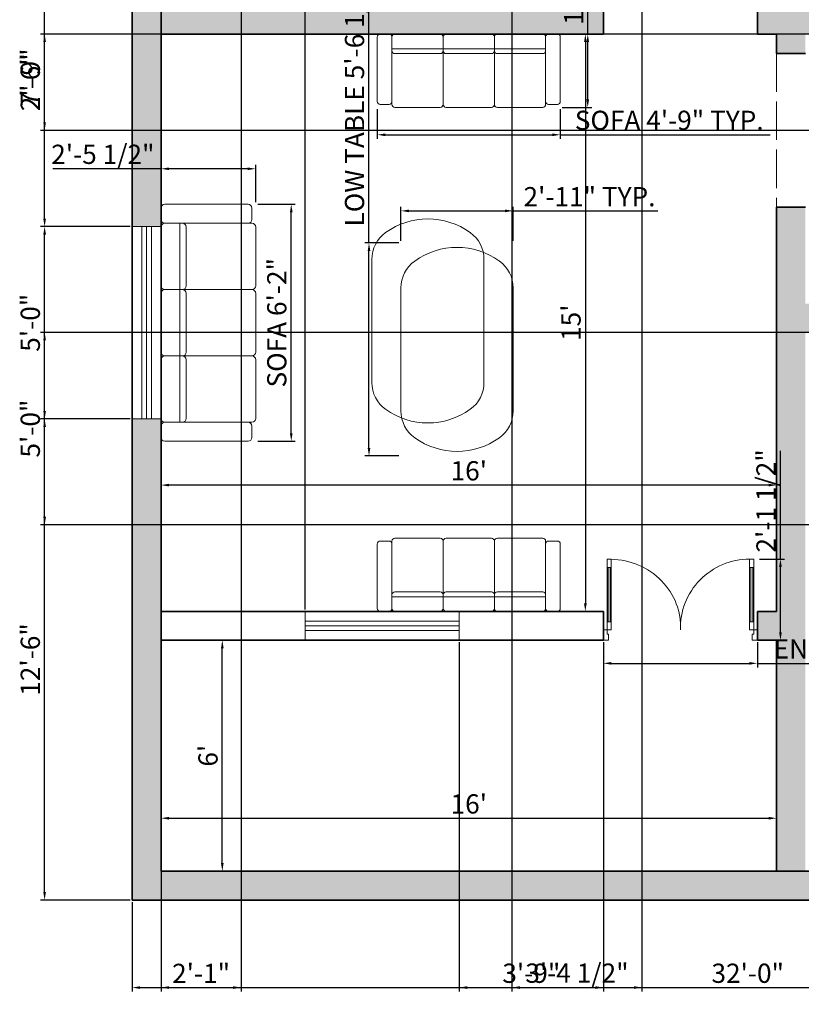
# Model space of a CAD drawing. Units: inches. Extents: x -40 to 424, y -33 to 568.
# Tile 1 of 8: x -35 to 209, y -33 to 275. Entities that reach past the tile are written whole.
import ezdxf

# ---------------------------------------------------------------- set-up
doc = ezdxf.new("R2010")
doc.units = ezdxf.units.IN
doc.linetypes.add('ACAD_ISO02W100', pattern=[15, 12, -3])
for name, color, linetype, lineweight in [('A-ANNO-DIMS', 7, 'Continuous', 18), ('A-DOOR', 7, 'Continuous', 18), ('A-FURN', 7, 'Continuous', 18), ('A-GLAZ', 7, 'Continuous', 18), ('A-WALL-OVHD', 7, 'ACAD_ISO02W100', 18), ('A-WALL-PATT', 30, 'Continuous', 13), ('wall', 7, 'Continuous', 35)]:
    doc.layers.add(name, color=color, linetype=linetype, lineweight=lineweight)
doc.styles.get("Standard").update_dxf_attribs({"font": 'arial.ttf'})
doc.dimstyles.new('ISO-25', dxfattribs={"dimtxt": 6, "dimasz": 2.5, "dimexe": 1.25, "dimexo": 0.625, "dimtad": 1, "dimdec": 1, "dimlunit": 3, "dimtxsty": 'Standard', "dimcen": 2.5, "dimadec": 0, "dimazin": 0, "dimtfac": 1, "dimtdec": 1, "dimtmove": 0, "dimatfit": 3, "dimfxl": 1, "dimarcsym": 0})

# ---------------------------------------------------------------- blocks, each defined once
blk = doc.blocks.new('A$C0A95752C')
for p, q in [((35, 710), (35, 790)), ((35, 790), (75, 790)), ((75, 790), (75, 710)), ((1425, 790), (1425, 710)), ((1465, 790), (1425, 790)), ((1465, 710), (1465, 790)), ((35, 710), (35, 180)), ((75, 710), (35, 710)), ((75, 710), (35, 710)), ((45, 710), (45, 180)), ((65, 710), (45, 710)), ((65, 180), (65, 710)), ((75, 180), (75, 710)), ((1425, 710), (1465, 710)), ((1425, 180), (1425, 710)), ((1425, 710), (1465, 710)), ((1435, 180), (1435, 710)), ((1435, 710), (1455, 710)), ((1455, 710), (1455, 180)), ((1465, 710), (1465, 180)), ((0, 100), (0, 0)), ((35, 100), (0, 100)), ((35, 180), (35, 100)), ((75, 180), (35, 180)), ((35, 180), (75, 180)), ((35, 100), (75, 100)), ((35, 60), (35, 100)), ((45, 180), (65, 180)), ((75, 100), (75, 180)), ((1465, 180), (1425, 180)), ((1425, 100), (1425, 180)), ((1425, 180), (1465, 180)), ((1465, 100), (1425, 100)), ((1455, 180), (1435, 180)), ((1465, 180), (1465, 100)), ((1465, 100), (1500, 100)), ((1465, 60), (1465, 100)), ((1500, 100), (1500, 0)), ((50, 60), (35, 60)), ((50, 50), (50, 60)), ((50, 0), (50, 50)), ((1450, 50), (1450, 60)), ((1450, 60), (1465, 60)), ((1450, 0), (1450, 50)), ((0, 0), (50, 0)), ((1500, 0), (1450, 0))]:
    blk.add_line(p, q)
blk.add_arc((1422.2, 117), 673, 89.76573, 181.44381)
blk.add_ellipse((73.9, 151.1), major_axis=(666.9, -121.7), ratio=0.940794, start_param=0.11153, end_param=1.73917)
blk = doc.blocks.new('A$C0513100E')
for p, q in [((0, 0.768), (0, 0.064)), ((0.032, 0.8), (0.128, 0.8)), ((0.16, 0.768), (0.16, 0.032)), ((0.688, 0.8), (0.192, 0.8)), ((0.72, 0.768), (0.72, 0.032)), ((1.248, 0.8), (0.752, 0.8)), ((1.28, 0.768), (1.28, 0.032)), ((1.808, 0.8), (1.312, 0.8)), ((1.84, 0.032), (1.84, 0.768)), ((1.872, 0.8), (1.968, 0.8)), ((2, 0.064), (2, 0.768)), ((0.72, 0.64), (0.16, 0.64)), ((0.688, 0.5867), (0.192, 0.5867)), ((1.28, 0.64), (0.72, 0.64)), ((1.248, 0.5867), (0.752, 0.5867)), ((1.84, 0.64), (1.28, 0.64)), ((1.808, 0.5867), (1.312, 0.5867)), ((0.72, 0.064), (0.72, 0.4017)), ((1.28, 0.064), (1.28, 0.4017)), ((1.84, 0.064), (1.84, 0.4017)), ((0.032, 0.032), (0.128, 0.032)), ((0.192, 0), (0.688, 0)), ((0.752, 0), (1.248, 0)), ((1.312, 0), (1.808, 0)), ((1.872, 0.032), (1.968, 0.032))]:
    blk.add_line(p, q)
for centre, start, end in [((0.032, 0.768), 90, 180), ((0.128, 0.768), 0, 90), ((0.192, 0.768), 90, 180), ((0.688, 0.768), 0, 90), ((0.752, 0.768), 90, 180), ((1.248, 0.768), 0, 90), ((1.312, 0.768), 90, 180), ((1.808, 0.768), 0, 90), ((1.872, 0.768), 90, 180), ((1.968, 0.768), 0, 90), ((0.192, 0.6187), 180, 270), ((0.688, 0.6187), 270, 0), ((0.752, 0.6187), 180, 270), ((1.248, 0.6187), 270, 0), ((1.312, 0.6187), 180, 270), ((1.808, 0.6187), 270, 0), ((0.032, 0.064), 180, 270), ((0.128, 0.064), 270, 0), ((0.192, 0.032), 180, 270), ((0.688, 0.032), 270, 0), ((0.752, 0.032), 180, 270), ((1.248, 0.032), 270, 0), ((1.312, 0.032), 180, 270), ((1.808, 0.032), 270, 0), ((1.872, 0.064), 180, 270), ((1.968, 0.064), 270, 0)]:
    blk.add_arc(centre, 0.032, start, end)
blk = doc.blocks.new('*D17')
at = {"layer": 'A-ANNO-DIMS', "color": 0, "lineweight": -2, "transparency": 16777216}
for p, q in [((9.63, 81), (29.37, 81)), ((28.12, 11.5), (28.12, 78.5)), ((9.63, 9), (29.37, 9))]:
    blk.add_line(p, q, dxfattribs=at)
at = {"layer": 'A-ANNO-DIMS', "color": 0, "transparency": 16777216}
for points in [[(27.71, 78.5), (28.54, 78.5), (28.12, 81)], [(27.71, 11.5), (28.54, 11.5), (28.12, 9)]]:
    blk.add_solid(points, dxfattribs=at)
at = {"layer": 'Defpoints', "color": 0, "transparency": 16777216}
for p in [(9, 81), (28.12, 81), (9, 9)]:
    blk.add_point(p, dxfattribs=at)
at = {"layer": 'A-ANNO-DIMS', "color": 0, "transparency": 16777216, "insert": (24.43, 45), "char_height": 6, "attachment_point": 5, "rotation": 90}
blk.add_mtext("6'", dxfattribs=at)
blk = doc.blocks.new('*D18')
at = {"layer": 'A-ANNO-DIMS', "color": 0, "lineweight": -2, "transparency": 16777216}
for p, q in [((9, 33.09), (9, 24.25)), ((201, 31.04), (201, 24.25)), ((11.5, 25.5), (198.5, 25.5))]:
    blk.add_line(p, q, dxfattribs=at)
at = {"layer": 'A-ANNO-DIMS', "color": 0, "transparency": 16777216}
for points in [[(11.5, 25.92), (11.5, 25.08), (9, 25.5)], [(198.5, 25.92), (198.5, 25.08), (201, 25.5)]]:
    blk.add_solid(points, dxfattribs=at)
at = {"layer": 'Defpoints', "color": 0, "transparency": 16777216}
for p in [(9, 33.71), (201, 31.66), (201, 25.5)]:
    blk.add_point(p, dxfattribs=at)
at = {"layer": 'A-ANNO-DIMS', "color": 0, "transparency": 16777216, "insert": (105, 29.19), "char_height": 6, "attachment_point": 5}
blk.add_mtext("16'", dxfattribs=at)
blk = doc.blocks.new('*D23')
at = {"layer": 'A-ANNO-DIMS', "color": 0, "lineweight": -2, "transparency": 16777216}
for p, q in [((9, 132.5), (9, 128.12)), ((201, 132.5), (201, 128.12)), ((198.5, 129.37), (11.5, 129.37))]:
    blk.add_line(p, q, dxfattribs=at)
at = {"layer": 'A-ANNO-DIMS', "color": 0, "transparency": 16777216}
for points in [[(11.5, 129.79), (11.5, 128.96), (9, 129.37)], [(198.5, 129.79), (198.5, 128.96), (201, 129.37)]]:
    blk.add_solid(points, dxfattribs=at)
at = {"layer": 'Defpoints', "color": 0, "transparency": 16777216}
for p in [(9, 133.12), (201, 133.12), (9, 129.37)]:
    blk.add_point(p, dxfattribs=at)
at = {"layer": 'A-ANNO-DIMS', "color": 0, "transparency": 16777216, "insert": (105, 133.06), "char_height": 6, "attachment_point": 5}
blk.add_mtext("16'", dxfattribs=at)
blk = doc.blocks.new('*D24')
at = {"layer": 'A-ANNO-DIMS', "color": 0, "lineweight": -2, "transparency": 16777216}
for p, q in [((146.38, 270), (140.1, 270)), ((141.35, 267.5), (141.35, 92.5)), ((142.23, 90), (140.1, 90))]:
    blk.add_line(p, q, dxfattribs=at)
at = {"layer": 'A-ANNO-DIMS', "color": 0, "transparency": 16777216}
for points in [[(140.94, 267.5), (141.77, 267.5), (141.35, 270)], [(140.94, 92.5), (141.77, 92.5), (141.35, 90)]]:
    blk.add_solid(points, dxfattribs=at)
at = {"layer": 'Defpoints', "color": 0, "transparency": 16777216}
for p in [(147, 270), (141.35, 90), (142.85, 90)]:
    blk.add_point(p, dxfattribs=at)
at = {"layer": 'A-ANNO-DIMS', "color": 0, "transparency": 16777216, "insert": (137.67, 180), "char_height": 6, "attachment_point": 5, "rotation": 90}
blk.add_mtext("15'", dxfattribs=at)
blk = doc.blocks.new('WIN-48IN')
for p, q in [((0, 0), (0, 9)), ((48, 0), (48, 9)), ((0, 6), (48, 6)), ((0, 4.5), (48, 4.5)), ((0, 3), (48, 3))]:
    blk.add_line(p, q)
blk = doc.blocks.new('TABLE-LOW-OBLONG')
for points in [[(35, 20.37), (35, 50.99, 0.241531), (30.71, 59.36, 0.321887), (4.29, 59.36, 0.241531), (0, 50.99), (0, 20.37)], [(35, 43.24), (35, 12.61, -0.241531), (30.71, 4.25, -0.321887), (4.29, 4.25, -0.241531), (0, 12.61), (0, 43.24)]]:
    blk.add_lwpolyline(points, format="xyb")
blk = doc.blocks.new('*D51')
at = {"layer": 'A-ANNO-DIMS', "color": 0, "lineweight": -2, "transparency": 16777216}
for p, q in [((147, 80.37), (147, 72.55)), ((195, 80.37), (195, 72.55)), ((149.5, 73.8), (192.5, 73.8)), ((195, 73.8), (272.6, 73.8))]:
    blk.add_line(p, q, dxfattribs=at)
at = {"layer": 'A-ANNO-DIMS', "color": 0, "transparency": 16777216}
for points in [[(149.5, 74.22), (149.5, 73.38), (147, 73.8)], [(192.5, 74.22), (192.5, 73.38), (195, 73.8)]]:
    blk.add_solid(points, dxfattribs=at)
at = {"layer": 'Defpoints', "color": 0, "transparency": 16777216}
for p in [(147, 81), (195, 81), (195, 73.8)]:
    blk.add_point(p, dxfattribs=at)
at = {"layer": 'A-ANNO-DIMS', "color": 0, "transparency": 16777216, "insert": (235.05, 77.53), "char_height": 6, "attachment_point": 5}
blk.add_mtext('ENTRY DOOR 4\'-0"', dxfattribs=at)
blk = doc.blocks.new('*D52')
at = {"layer": 'A-ANNO-DIMS', "color": 0, "lineweight": -2, "transparency": 16777216}
for p, q in [((202.2, 106.3), (202.2, 140.09)), ((195.63, 106.3), (203.45, 106.3)), ((202.2, 83.5), (202.2, 103.8)), ((195.63, 81), (203.45, 81))]:
    blk.add_line(p, q, dxfattribs=at)
at = {"layer": 'A-ANNO-DIMS', "color": 0, "transparency": 16777216}
for points in [[(201.78, 103.8), (202.62, 103.8), (202.2, 106.3)], [(201.78, 83.5), (202.62, 83.5), (202.2, 81)]]:
    blk.add_solid(points, dxfattribs=at)
at = {"layer": 'Defpoints', "color": 0, "transparency": 16777216}
for p in [(195, 106.3), (202.2, 106.3), (195, 81)]:
    blk.add_point(p, dxfattribs=at)
at = {"layer": 'A-ANNO-DIMS', "color": 0, "transparency": 16777216, "insert": (198.47, 124.45), "char_height": 6, "attachment_point": 5, "rotation": 90}
blk.add_mtext('2\'-1 1/2"', dxfattribs=at)
blk = doc.blocks.new('*D53')
at = {"layer": 'A-ANNO-DIMS', "color": 0, "lineweight": -2, "transparency": 16777216}
for p, q in [((39.17, 216.93), (50.87, 216.93)), ((49.62, 145.57), (49.62, 214.43)), ((39.17, 143.07), (50.87, 143.07))]:
    blk.add_line(p, q, dxfattribs=at)
at = {"layer": 'A-ANNO-DIMS', "color": 0, "transparency": 16777216}
for points in [[(49.21, 214.43), (50.04, 214.43), (49.62, 216.93)], [(49.21, 145.57), (50.04, 145.57), (49.62, 143.07)]]:
    blk.add_solid(points, dxfattribs=at)
at = {"layer": 'Defpoints', "color": 0, "transparency": 16777216}
for p in [(38.54, 216.93), (49.62, 216.93), (38.54, 143.07)]:
    blk.add_point(p, dxfattribs=at)
at = {"layer": 'A-ANNO-DIMS', "color": 0, "transparency": 16777216, "insert": (45.89, 180), "char_height": 6, "attachment_point": 5, "rotation": 90}
blk.add_mtext('SOFA 6\'-2"', dxfattribs=at)
blk = doc.blocks.new('*D54')
at = {"layer": 'A-ANNO-DIMS', "color": 0, "lineweight": -2, "transparency": 16777216}
for p, q in [((9, 228.01), (-24.78, 228.01)), ((9, 217.55), (9, 229.26)), ((36.04, 228.01), (11.5, 228.01)), ((38.54, 217.55), (38.54, 229.26))]:
    blk.add_line(p, q, dxfattribs=at)
at = {"layer": 'A-ANNO-DIMS', "color": 0, "transparency": 16777216}
for points in [[(11.5, 228.42), (11.5, 227.59), (9, 228.01)], [(36.04, 228.42), (36.04, 227.59), (38.54, 228.01)]]:
    blk.add_solid(points, dxfattribs=at)
at = {"layer": 'Defpoints', "color": 0, "transparency": 16777216}
for p in [(9, 228.01), (9, 216.93), (38.54, 216.93)]:
    blk.add_point(p, dxfattribs=at)
at = {"layer": 'A-ANNO-DIMS', "color": 0, "transparency": 16777216, "insert": (-9.14, 231.74), "char_height": 6, "attachment_point": 5}
blk.add_mtext('2\'-5 1/2"', dxfattribs=at)
blk = doc.blocks.new('*D55')
at = {"layer": 'A-ANNO-DIMS', "color": 0, "lineweight": -2, "transparency": 16777216}
for p, q in [((76.46, 246.55), (76.46, 237.36)), ((133.54, 246.55), (133.54, 237.36)), ((78.96, 238.61), (131.04, 238.61)), ((133.54, 238.61), (198.98, 238.61))]:
    blk.add_line(p, q, dxfattribs=at)
at = {"layer": 'A-ANNO-DIMS', "color": 0, "transparency": 16777216}
for points in [[(78.96, 239.03), (78.96, 238.19), (76.46, 238.61)], [(131.04, 239.03), (131.04, 238.19), (133.54, 238.61)]]:
    blk.add_solid(points, dxfattribs=at)
at = {"layer": 'Defpoints', "color": 0, "transparency": 16777216}
for p in [(76.46, 247.17), (133.54, 247.17), (133.54, 238.61)]:
    blk.add_point(p, dxfattribs=at)
at = {"layer": 'A-ANNO-DIMS', "color": 0, "transparency": 16777216, "insert": (167.51, 242.34), "char_height": 6, "attachment_point": 5}
blk.add_mtext('SOFA 4\'-9" TYP.', dxfattribs=at)
blk = doc.blocks.new('*D56')
at = {"layer": 'A-ANNO-DIMS', "color": 0, "lineweight": -2, "transparency": 16777216}
for p, q in [((142.1, 270), (142.1, 314.42)), ((134.16, 270), (143.35, 270)), ((142.1, 249.67), (142.1, 267.5)), ((134.16, 247.17), (143.35, 247.17))]:
    blk.add_line(p, q, dxfattribs=at)
at = {"layer": 'A-ANNO-DIMS', "color": 0, "transparency": 16777216}
for points in [[(141.68, 267.5), (142.51, 267.5), (142.1, 270)], [(141.68, 249.67), (142.51, 249.67), (142.1, 247.17)]]:
    blk.add_solid(points, dxfattribs=at)
at = {"layer": 'Defpoints', "color": 0, "transparency": 16777216}
for p in [(133.54, 270), (142.1, 270), (133.54, 247.17)]:
    blk.add_point(p, dxfattribs=at)
at = {"layer": 'A-ANNO-DIMS', "color": 0, "transparency": 16777216, "insert": (138.46, 293.46), "char_height": 6, "attachment_point": 5, "rotation": 90}
blk.add_mtext('1\'-11" TYP.', dxfattribs=at)
blk = doc.blocks.new('*D59')
at = {"layer": 'A-ANNO-DIMS', "color": 0, "lineweight": -2, "transparency": 16777216}
for p, q in [((73.87, 204.92), (73.87, 309.26)), ((83.22, 204.92), (72.62, 204.92)), ((73.87, 140.98), (73.87, 202.42)), ((83.22, 138.48), (72.62, 138.48))]:
    blk.add_line(p, q, dxfattribs=at)
at = {"layer": 'A-ANNO-DIMS', "color": 0, "transparency": 16777216}
for points in [[(73.46, 202.42), (74.29, 202.42), (73.87, 204.92)], [(73.46, 140.98), (74.29, 140.98), (73.87, 138.48)]]:
    blk.add_solid(points, dxfattribs=at)
at = {"layer": 'Defpoints', "color": 0, "transparency": 16777216}
for p in [(73.87, 204.92), (83.84, 204.92), (83.84, 138.48)]:
    blk.add_point(p, dxfattribs=at)
at = {"layer": 'A-ANNO-DIMS', "color": 0, "transparency": 16777216, "insert": (70.14, 258.34), "char_height": 6, "attachment_point": 5, "rotation": 90}
blk.add_mtext('LOW TABLE 5\'-6 1/2" TYP.', dxfattribs=at)
blk = doc.blocks.new('*D60')
at = {"layer": 'A-ANNO-DIMS', "color": 0, "lineweight": -2, "transparency": 16777216}
for p, q in [((83.84, 205.55), (83.84, 216.14)), ((118.84, 205.55), (118.84, 216.14)), ((86.34, 214.89), (116.34, 214.89)), ((118.84, 214.89), (163.93, 214.89))]:
    blk.add_line(p, q, dxfattribs=at)
at = {"layer": 'A-ANNO-DIMS', "color": 0, "transparency": 16777216}
for points in [[(86.34, 215.3), (86.34, 214.47), (83.84, 214.89)], [(116.34, 215.3), (116.34, 214.47), (118.84, 214.89)]]:
    blk.add_solid(points, dxfattribs=at)
at = {"layer": 'Defpoints', "color": 0, "transparency": 16777216}
for p in [(118.84, 214.89), (83.84, 204.92), (118.84, 204.92)]:
    blk.add_point(p, dxfattribs=at)
at = {"layer": 'A-ANNO-DIMS', "color": 0, "transparency": 16777216, "insert": (142.64, 218.53), "char_height": 6, "attachment_point": 5}
blk.add_mtext('2\'-11" TYP.', dxfattribs=at)
blk = doc.blocks.new('*D79')
at = {"layer": 'A-ANNO-DIMS', "color": 0, "lineweight": -2, "transparency": 16777216}
for p, q in [((0, -0.62), (0, -28.55)), ((384, -0.62), (384, -28.55)), ((2.5, -27.3), (381.5, -27.3))]:
    blk.add_line(p, q, dxfattribs=at)
at = {"layer": 'A-ANNO-DIMS', "color": 0, "transparency": 16777216}
for points in [[(2.5, -26.88), (2.5, -27.72), (0, -27.3)], [(381.5, -26.88), (381.5, -27.72), (384, -27.3)]]:
    blk.add_solid(points, dxfattribs=at)
at = {"layer": 'Defpoints', "color": 0, "transparency": 16777216}
for p in [(0, 0), (384, 0), (384, -27.3)]:
    blk.add_point(p, dxfattribs=at)
at = {"layer": 'A-ANNO-DIMS', "color": 0, "transparency": 16777216, "insert": (192, -23.61), "char_height": 6, "attachment_point": 5}
blk.add_mtext('32\'-0"', dxfattribs=at)
blk = doc.blocks.new('*D81')
at = {"layer": 'A-ANNO-DIMS', "color": 0, "lineweight": -2, "transparency": 16777216}
for p, q in [((-0.63, 210), (-28.55, 210)), ((-27.3, 152.5), (-27.3, 207.5)), ((-0.63, 150), (-28.55, 150))]:
    blk.add_line(p, q, dxfattribs=at)
at = {"layer": 'A-ANNO-DIMS', "color": 0, "transparency": 16777216}
for points in [[(-27.72, 207.5), (-26.88, 207.5), (-27.3, 210)], [(-27.72, 152.5), (-26.88, 152.5), (-27.3, 150)]]:
    blk.add_solid(points, dxfattribs=at)
at = {"layer": 'Defpoints', "color": 0, "transparency": 16777216}
for p in [(-27.3, 210), (0, 210), (0, 150)]:
    blk.add_point(p, dxfattribs=at)
at = {"layer": 'A-ANNO-DIMS', "color": 0, "transparency": 16777216, "insert": (-30.99, 180), "char_height": 6, "attachment_point": 5, "rotation": 90}
blk.add_mtext('5\'-0"', dxfattribs=at)
blk = doc.blocks.new('*D82')
at = {"layer": 'A-ANNO-DIMS', "color": 0, "lineweight": -2, "transparency": 16777216}
for p, q in [((-0.63, 150), (-28.55, 150)), ((-27.3, 2.5), (-27.3, 147.5)), ((-0.63, 0), (-28.55, 0))]:
    blk.add_line(p, q, dxfattribs=at)
at = {"layer": 'A-ANNO-DIMS', "color": 0, "transparency": 16777216}
for points in [[(-27.72, 147.5), (-26.88, 147.5), (-27.3, 150)], [(-27.72, 2.5), (-26.88, 2.5), (-27.3, 0)]]:
    blk.add_solid(points, dxfattribs=at)
at = {"layer": 'Defpoints', "color": 0, "transparency": 16777216}
for p in [(-27.3, 150), (0, 150), (0, 0)]:
    blk.add_point(p, dxfattribs=at)
at = {"layer": 'A-ANNO-DIMS', "color": 0, "transparency": 16777216, "insert": (-30.99, 75), "char_height": 6, "attachment_point": 5, "rotation": 90}
blk.add_mtext('12\'-6"', dxfattribs=at)
blk = doc.blocks.new('*D83')
at = {"layer": 'A-ANNO-DIMS', "color": 0, "lineweight": -2, "transparency": 16777216}
for p, q in [((-0.63, 303), (-28.55, 303)), ((-27.3, 212.5), (-27.3, 300.5)), ((-0.63, 210), (-28.55, 210))]:
    blk.add_line(p, q, dxfattribs=at)
at = {"layer": 'A-ANNO-DIMS', "color": 0, "transparency": 16777216}
for points in [[(-27.72, 300.5), (-26.88, 300.5), (-27.3, 303)], [(-27.72, 212.5), (-26.88, 212.5), (-27.3, 210)]]:
    blk.add_solid(points, dxfattribs=at)
at = {"layer": 'Defpoints', "color": 0, "transparency": 16777216}
for p in [(-27.3, 303), (0, 303), (0, 210)]:
    blk.add_point(p, dxfattribs=at)
at = {"layer": 'A-ANNO-DIMS', "color": 0, "transparency": 16777216, "insert": (-30.99, 256.5), "char_height": 6, "attachment_point": 5, "rotation": 90}
blk.add_mtext('7\'-9"', dxfattribs=at)
blk = doc.blocks.new('*D87')
at = {"layer": 'A-ANNO-DIMS', "color": 0, "lineweight": -2, "transparency": 16777216}
for p, q in [((374.38, 177), (-28.55, 177)), ((-27.3, 119.5), (-27.3, 174.5)), ((374.38, 117), (-28.55, 117))]:
    blk.add_line(p, q, dxfattribs=at)
at = {"layer": 'A-ANNO-DIMS', "color": 0, "transparency": 16777216}
for points in [[(-27.72, 174.5), (-26.88, 174.5), (-27.3, 177)], [(-27.72, 119.5), (-26.88, 119.5), (-27.3, 117)]]:
    blk.add_solid(points, dxfattribs=at)
at = {"layer": 'Defpoints', "color": 0, "transparency": 16777216}
for p in [(-27.3, 177), (375, 177), (375, 117)]:
    blk.add_point(p, dxfattribs=at)
at = {"layer": 'A-ANNO-DIMS', "color": 0, "transparency": 16777216, "insert": (-30.99, 147), "char_height": 6, "attachment_point": 5, "rotation": 90}
blk.add_mtext('5\'-0"', dxfattribs=at)
blk = doc.blocks.new('*D88')
at = {"layer": 'A-ANNO-DIMS', "color": 0, "lineweight": -2, "transparency": 16777216}
for p, q in [((374.38, 270), (-28.55, 270)), ((-27.3, 242.5), (-27.3, 267.5)), ((374.38, 240), (-28.55, 240))]:
    blk.add_line(p, q, dxfattribs=at)
at = {"layer": 'A-ANNO-DIMS', "color": 0, "transparency": 16777216}
for points in [[(-27.72, 267.5), (-26.88, 267.5), (-27.3, 270)], [(-27.72, 242.5), (-26.88, 242.5), (-27.3, 240)]]:
    blk.add_solid(points, dxfattribs=at)
at = {"layer": 'Defpoints', "color": 0, "transparency": 16777216}
for p in [(-27.3, 270), (375, 270), (375, 240)]:
    blk.add_point(p, dxfattribs=at)
at = {"layer": 'A-ANNO-DIMS', "color": 0, "transparency": 16777216, "insert": (-30.99, 255), "char_height": 6, "attachment_point": 5, "rotation": 90}
blk.add_mtext('2\'-6"', dxfattribs=at)
blk = doc.blocks.new('*D90')
at = {"layer": 'A-ANNO-DIMS', "color": 0, "lineweight": -2, "transparency": 16777216}
for p, q in [((102, 80.37), (102, -28.55)), ((147, 80.37), (147, -28.55)), ((104.5, -27.3), (144.5, -27.3))]:
    blk.add_line(p, q, dxfattribs=at)
at = {"layer": 'A-ANNO-DIMS', "color": 0, "transparency": 16777216}
for points in [[(104.5, -26.88), (104.5, -27.72), (102, -27.3)], [(144.5, -26.88), (144.5, -27.72), (147, -27.3)]]:
    blk.add_solid(points, dxfattribs=at)
at = {"layer": 'Defpoints', "color": 0, "transparency": 16777216}
for p in [(102, 81), (147, 81), (147, -27.3)]:
    blk.add_point(p, dxfattribs=at)
at = {"layer": 'A-ANNO-DIMS', "color": 0, "transparency": 16777216, "insert": (124.5, -23.61), "char_height": 6, "attachment_point": 5}
blk.add_mtext('3\'-9"', dxfattribs=at)
blk = doc.blocks.new('*D91')
at = {"layer": 'A-ANNO-DIMS', "color": 0, "lineweight": -2, "transparency": 16777216}
for p, q in [((9, 90.62), (9, 556.55)), ((54, 90.62), (54, 556.55)), ((11.5, 555.3), (51.5, 555.3))]:
    blk.add_line(p, q, dxfattribs=at)
at = {"layer": 'A-ANNO-DIMS', "color": 0, "transparency": 16777216}
for points in [[(11.5, 555.72), (11.5, 554.88), (9, 555.3)], [(51.5, 555.72), (51.5, 554.88), (54, 555.3)]]:
    blk.add_solid(points, dxfattribs=at)
at = {"layer": 'Defpoints', "color": 0, "transparency": 16777216}
for p in [(54, 555.3), (9, 90), (54, 90)]:
    blk.add_point(p, dxfattribs=at)
at = {"layer": 'A-ANNO-DIMS', "color": 0, "transparency": 16777216, "insert": (31.5, 558.99), "char_height": 6, "attachment_point": 5}
blk.add_mtext('3\'-9"', dxfattribs=at)
blk = doc.blocks.new('*D92')
at = {"layer": 'A-ANNO-DIMS', "color": 0, "lineweight": -2, "transparency": 16777216}
for p, q in [((118.47, 470.38), (118.47, -28.55)), ((159, 470.38), (159, -28.55)), ((120.97, -27.3), (156.5, -27.3))]:
    blk.add_line(p, q, dxfattribs=at)
at = {"layer": 'A-ANNO-DIMS', "color": 0, "transparency": 16777216}
for points in [[(120.97, -26.88), (120.97, -27.72), (118.47, -27.3)], [(156.5, -26.88), (156.5, -27.72), (159, -27.3)]]:
    blk.add_solid(points, dxfattribs=at)
at = {"layer": 'Defpoints', "color": 0, "transparency": 16777216}
for p in [(118.47, 471), (159, 471), (159, -27.3)]:
    blk.add_point(p, dxfattribs=at)
at = {"layer": 'A-ANNO-DIMS', "color": 0, "transparency": 16777216, "insert": (138.73, -23.57), "char_height": 6, "attachment_point": 5}
blk.add_mtext('3\'-4 1/2"', dxfattribs=at)
blk = doc.blocks.new('*D101')
at = {"layer": 'A-ANNO-DIMS', "color": 0, "lineweight": -2, "transparency": 16777216}
for p, q in [((9, 357.82), (9, -28.55)), ((34, 357.82), (34, -28.55)), ((11.5, -27.3), (31.5, -27.3))]:
    blk.add_line(p, q, dxfattribs=at)
at = {"layer": 'A-ANNO-DIMS', "color": 0, "transparency": 16777216}
for points in [[(11.5, -26.88), (11.5, -27.72), (9, -27.3)], [(31.5, -26.88), (31.5, -27.72), (34, -27.3)]]:
    blk.add_solid(points, dxfattribs=at)
at = {"layer": 'Defpoints', "color": 0, "transparency": 16777216}
for p in [(9, 358.44), (34, 358.44), (34, -27.3)]:
    blk.add_point(p, dxfattribs=at)
at = {"layer": 'A-ANNO-DIMS', "color": 0, "transparency": 16777216, "insert": (21.5, -23.66), "char_height": 6, "attachment_point": 5}
blk.add_mtext('2\'-1"', dxfattribs=at)

msp = doc.modelspace()

# ---------------------------------------------------------------- hatches: boundary and pattern name
at = {"layer": 'A-WALL-PATT'}
h = msp.add_hatch(color=256, dxfattribs=at)
h.dxf.hatch_style = 1
h.paths.add_polyline_path([(9, 399), (0, 399), (0, 351), (9, 351)])
h.paths.add_polyline_path([(9, 303), (0, 303), (0, 210), (9, 210)])
h.paths.add_polyline_path([(9, 150), (0, 150), (0, 0), (384, 0), (384, 69), (375, 69), (375, 62.24), (375, 9), (9, 9)])
h.paths.add_polyline_path([(210, 177), (216, 177), (216, 186), (210, 186), (210, 216), (201, 216), (201, 90), (195, 90), (195, 81), (201, 81), (201, 9), (210, 9)])
h.paths.add_polyline_path([(384, 216), (375, 216), (375, 117), (384, 117)])
h.paths.add_polyline_path([(384, 298.5), (375, 298.5), (375, 279), (375, 240), (384, 240)])
h.paths.add_polyline_path([(384, 417), (375, 417), (375, 334.5), (384, 334.5)])
h.paths.add_polyline_path([(384, 528), (216, 528), (216, 519), (375, 519), (375, 465), (384, 465)])
h.paths.add_polyline_path([(192, 528), (0, 528), (0, 511.5), (9, 511.5), (9, 519), (192, 519)])
h.paths.add_polyline_path([(9, 487.5), (0, 487.5), (0, 447), (9, 447)])
h.paths.add_polyline_path([(111, 480), (9, 480), (9, 471), (111, 471)])
h.paths.add_polyline_path([(174, 519), (165, 519), (165, 354), (174, 354)])
h.paths.add_polyline_path([(243, 426), (237.86, 426), (234, 426), (234, 420), (174, 420), (174, 411), (234, 411), (234, 405), (239.14, 405), (243, 405)])
h.paths.add_polyline_path([(243, 519), (234, 519), (234, 460.14, -0.031638), (237.86, 460.2), (237.86, 462), (243, 462)])
h.paths.add_polyline_path([(243, 369), (234, 369), (234, 354), (375, 354), (375, 363), (243, 363)])
h.paths.add_polyline_path([(375, 279), (195, 279), (195, 270), (201, 270), (201, 264), (210, 264), (210, 270), (375, 270)])
h.paths.add_polyline_path([(291, 270), (282, 270), (282, 222), (286.29, 222), (291, 222)])
h.paths.add_polyline_path([(375, 186), (291, 186), (291, 192), (282, 192), (282, 186), (252, 186), (252, 180.86), (252, 177), (375, 177)])
h.paths.add_polyline_path([(147, 279), (9, 279), (9, 270), (147, 270)])

# ---------------------------------------------------------------- linework, layer by layer
at = {"layer": 'A-GLAZ'}
for p, q in [((0, 210), (9, 210)), ((3, 210), (3, 150)), ((4.5, 210), (4.5, 150)), ((6, 210), (6, 150)), ((0, 150), (9, 150))]:
    msp.add_line(p, q, dxfattribs=at)
at = {"layer": 'A-WALL-OVHD'}
for p, q in [((195, 270), (147, 270)), ((201, 264), (201, 216))]:
    msp.add_line(p, q, dxfattribs=at)
at = {"layer": 'wall'}
for p, q in [((9, 519), (9, 9)), ((147, 279), (147, 270)), ((195, 279), (195, 270)), ((9, 270), (147, 270)), ((195, 270), (201, 270)), ((201, 270), (201, 264)), ((201, 264), (210, 264)), ((201, 216), (210, 216)), ((201, 216), (201, 90)), ((9, 90), (147, 90)), ((147, 90), (147, 81)), ((195, 90), (195, 81)), ((195, 90), (201, 90)), ((9, 81), (147, 81)), ((195, 81), (201, 81)), ((201, 81), (201, 9)), ((9, 9), (375, 9))]:
    msp.add_line(p, q, dxfattribs=at)
msp.add_lwpolyline([(0, 0), (384, 0), (384, 528), (0, 528)], close=True, dxfattribs=at)

# ---------------------------------------------------------------- block references
at = {"layer": 'A-DOOR', "xscale": 0.032, "yscale": 0.032, "zscale": 0.032}
msp.add_blockref('A$C0A95752C', (147, 81), dxfattribs=at)
at = {"layer": 'A-FURN', "xscale": 28.53662023476671, "yscale": 28.53662023476671, "zscale": 28.53662023476671}
msp.add_blockref('A$C0513100E', (76.46, 247.17), dxfattribs=at)
at = {"layer": 'A-FURN'}
for p, xscale, yscale, zscale, rotation in [((38.54, 143.07), 36.9291377736036, 36.9291377736036, 36.9291377736036, 90), ((76.46, 112.83), -28.53662023476671, 28.53662023476671, 28.53662023476671, 180)]:
    msp.add_blockref('A$C0513100E', p, dxfattribs=dict(at, xscale=xscale, yscale=yscale, zscale=zscale, rotation=rotation))
for p in [(74.74, 148.76), (83.84, 139.89)]:
    msp.add_blockref('TABLE-LOW-OBLONG', p, dxfattribs=at)
at = {"layer": 'A-GLAZ'}
msp.add_blockref('WIN-48IN', (54, 81), dxfattribs=at)

# ---------------------------------------------------------------- dimensions: what is measured, and where the dimension line sits
at = {"layer": 'A-ANNO-DIMS'}
for base, p1, p2, override, picture, middle in [((54, 555.3), (9, 90), (54, 90), {"dimdec": 1, "dimlfac": 1, "dimrnd": 0, "dimzin": 1, "dimdsep": 46, "dimlunit": 4, "dimfrac": 2}, '*D91', (31.5, 558.99)), ((159, -27.3), (118.47, 471), (159, 471), {"dimdec": 1, "dimlfac": 1, "dimrnd": 0, "dimzin": 1, "dimdsep": 46, "dimlunit": 4, "dimfrac": 2}, '*D92', (138.73, -23.57)), ((34, -27.3), (9, 358.44), (34, 358.44), {"dimdec": 1, "dimlfac": 1, "dimrnd": 0, "dimzin": 1, "dimdsep": 46, "dimlunit": 4, "dimfrac": 2}, '*D101', (21.5, -23.66)), ((147, -27.3), (102, 81), (147, 81), {"dimdec": 1, "dimlfac": 1, "dimrnd": 0, "dimzin": 1, "dimdsep": 46, "dimlunit": 4, "dimfrac": 2}, '*D90', (124.5, -23.61)), ((201, 25.5), (9, 33.71), (201, 31.66), {"dimclrd": 0, "dimclre": 0, "dimclrt": 0}, '*D18', (105, 29.19)), ((384, -27.3), (0, 0), (384, 0), {"dimdec": 1, "dimlfac": 1, "dimrnd": 0, "dimzin": 1, "dimdsep": 46, "dimlunit": 4, "dimfrac": 2}, '*D79', (192, -23.61))]:
    dim = msp.add_linear_dim(base=base, p1=p1, p2=p2, dimstyle='ISO-25', override=override, dxfattribs=at)
    dim.commit()
    dim.dimension.update_dxf_attribs({"geometry": picture, "text_midpoint": middle})
for base, p1, p2, text, picture, middle in [((142.1, 270), (133.54, 247.17), (133.54, 270), '<> TYP.', '*D56', (138.46, 293.46)), ((73.87, 204.92), (83.84, 138.48), (83.84, 204.92), 'LOW TABLE <> TYP.', '*D59', (70.14, 258.34)), ((49.62, 216.93), (38.54, 143.07), (38.54, 216.93), 'SOFA <>', '*D53', (45.89, 180))]:
    dim = msp.add_linear_dim(base=base, p1=p1, p2=p2, angle=90, text=text, dimstyle='ISO-25', override={"dimdec": 1, "dimlfac": 1, "dimrnd": 0, "dimzin": 1, "dimdsep": 46, "dimlunit": 4, "dimfrac": 2}, dxfattribs=at)
    dim.commit()
    dim.dimension.update_dxf_attribs({"geometry": picture, "text_midpoint": middle})
for base, p1, p2, angle, override, picture, middle in [((-27.3, 303), (0, 210), (0, 303), 90, {"dimdec": 1, "dimlfac": 1, "dimrnd": 0, "dimzin": 1, "dimdsep": 46, "dimlunit": 4, "dimfrac": 2}, '*D83', (-30.99, 256.5)), ((-27.3, 270), (375, 240), (375, 270), 90, {"dimdec": 1, "dimlfac": 1, "dimrnd": 0, "dimzin": 1, "dimdsep": 46, "dimlunit": 4, "dimfrac": 2}, '*D88', (-30.99, 255)), ((141.35, 90), (147, 270), (142.85, 90), 90, {"dimclrd": 0, "dimclre": 0, "dimclrt": 0}, '*D24', (137.67, 180)), ((9, 228.01), (38.54, 216.93), (9, 216.93), 180, {"dimdec": 1, "dimlfac": 1, "dimrnd": 0, "dimzin": 1, "dimdsep": 46, "dimlunit": 4, "dimfrac": 2}, '*D54', (-9.14, 231.74)), ((-27.3, 210), (0, 150), (0, 210), 90, {"dimdec": 1, "dimlfac": 1, "dimrnd": 0, "dimzin": 1, "dimdsep": 46, "dimlunit": 4, "dimfrac": 2}, '*D81', (-30.99, 180)), ((-27.3, 177), (375, 117), (375, 177), 90, {"dimdec": 1, "dimlfac": 1, "dimrnd": 0, "dimzin": 1, "dimdsep": 46, "dimlunit": 4, "dimfrac": 2}, '*D87', (-30.99, 147)), ((-27.3, 150), (0, 0), (0, 150), 90, {"dimdec": 1, "dimlfac": 1, "dimrnd": 0, "dimzin": 1, "dimdsep": 46, "dimlunit": 4, "dimfrac": 2}, '*D82', (-30.99, 75)), ((202.2, 106.3), (195, 81), (195, 106.3), 90, {"dimdec": 1, "dimlfac": 1, "dimrnd": 0, "dimzin": 1, "dimdsep": 46, "dimlunit": 4, "dimfrac": 2}, '*D52', (198.47, 124.45)), ((28.12, 81), (9, 9), (9, 81), 90, {"dimclrd": 0, "dimclre": 0, "dimclrt": 0}, '*D17', (24.43, 45))]:
    dim = msp.add_linear_dim(base=base, p1=p1, p2=p2, angle=angle, dimstyle='ISO-25', override=override, dxfattribs=at)
    dim.commit()
    dim.dimension.update_dxf_attribs({"geometry": picture, "text_midpoint": middle})
for base, p1, p2, text, picture, middle in [((133.54, 238.61), (76.46, 247.17), (133.54, 247.17), 'SOFA <> TYP.', '*D55', (167.51, 242.34)), ((118.84, 214.89), (83.84, 204.92), (118.84, 204.92), '<> TYP.', '*D60', (142.64, 218.53)), ((195, 73.8), (147, 81), (195, 81), 'ENTRY DOOR <>', '*D51', (235.05, 77.53))]:
    dim = msp.add_linear_dim(base=base, p1=p1, p2=p2, text=text, dimstyle='ISO-25', override={"dimdec": 1, "dimlfac": 1, "dimrnd": 0, "dimzin": 1, "dimdsep": 46, "dimlunit": 4, "dimfrac": 2}, dxfattribs=at)
    dim.commit()
    dim.dimension.update_dxf_attribs({"geometry": picture, "text_midpoint": middle})
dim = msp.add_linear_dim(base=(9, 129.37), p1=(201, 133.12), p2=(9, 133.12), dimstyle='ISO-25', override={"dimclrd": 0, "dimclre": 0, "dimclrt": 0}, dxfattribs=at)
dim.commit()
dim.dimension.update_dxf_attribs({"geometry": '*D23', "text_midpoint": (105, 129.37), "dimtype": 160})

doc.saveas('drawing.dxf')
